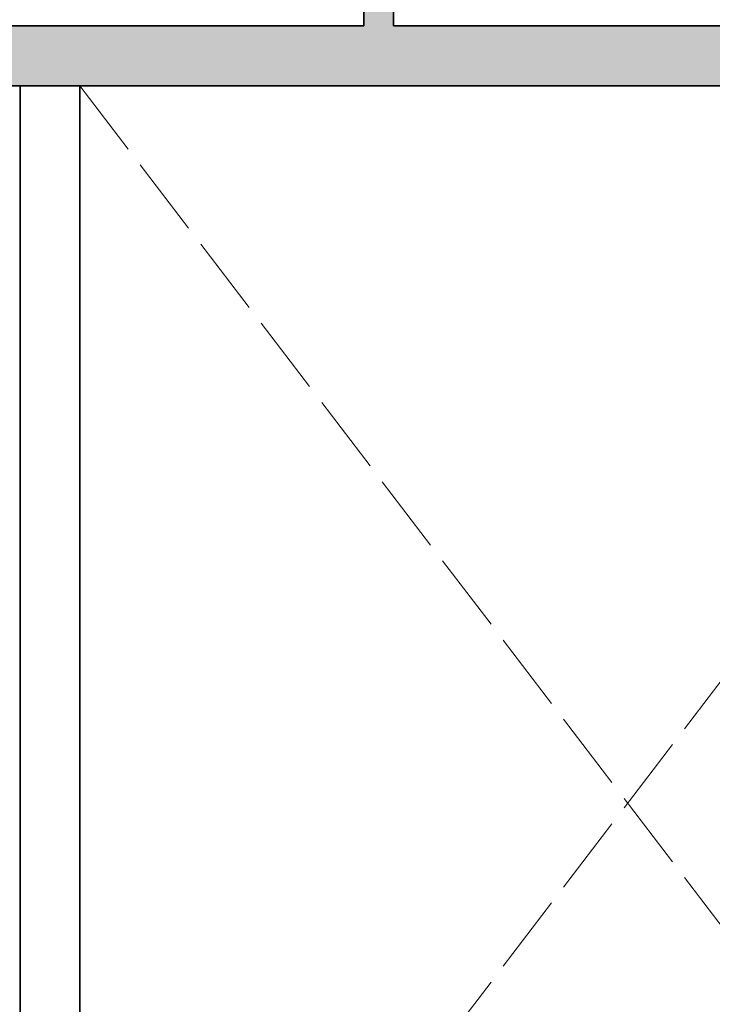
# Model space of a CAD drawing. Units: inches. Extents: x 2083 to 3317, y 1141 to 2115.
# Tile 252 of 256: x 2944 to 3048, y 1564 to 1713. Entities that reach past the tile are written whole.
import ezdxf

# ---------------------------------------------------------------- set-up
doc = ezdxf.new("R2010")
doc.units = ezdxf.units.IN
doc.linetypes.add('ACAD_ISO02W100', pattern=[15, 12, -3])
for name, color, linetype, lineweight in [('A-ANNO-DIMS', 2, 'Continuous', 18), ('A-FLOR-OPEN', 8, 'ACAD_ISO02W100', 13), ('A-WALL', 7, 'Continuous', 35)]:
    doc.layers.add(name, color=color, linetype=linetype, lineweight=lineweight)
doc.layers.add('A-WALL-PATT', color=251, linetype='Continuous', lineweight=13, true_color=0x636466)
doc.styles.get("Standard").update_dxf_attribs({"font": 'arial.ttf'})
doc.dimstyles.new('ISO-25', dxfattribs={"dimtxt": 12, "dimasz": 12, "dimexe": 1.25, "dimexo": 0.625, "dimtad": 1, "dimlunit": 3, "dimtxsty": 'Standard', "dimcen": 2.5, "dimadec": 0, "dimazin": 0, "dimtfac": 1, "dimtmove": 0, "dimatfit": 3, "dimfxl": 1, "dimarcsym": 0})

# ---------------------------------------------------------------- blocks, each defined once
blk = doc.blocks.new('*D71')
at = {"layer": 'A-ANNO-DIMS', "color": 0, "lineweight": -2, "transparency": 16777216}
for p, q in [((2997.14, 1794.66), (3020.88, 1769.53)), ((3093.61, 1692.52), (3029.12, 1760.8))]:
    blk.add_line(p, q, dxfattribs=at)
at = {"layer": 'A-ANNO-DIMS', "color": 0, "transparency": 16777216}
blk.add_solid([(3030.57, 1762.18), (3027.67, 1759.43), (3020.88, 1769.53)], dxfattribs=at)
at = {"layer": 'Defpoints', "color": 0, "transparency": 16777216}
for p in [(2997.14, 1794.66), (3020.88, 1769.53)]:
    blk.add_point(p, dxfattribs=at)
at = {"layer": 'A-ANNO-DIMS', "color": 0, "transparency": 16777216, "insert": (3070.45, 1726.99), "char_height": 12, "attachment_point": 5, "rotation": 313.3638}
blk.add_mtext('R2\'-10 1/2"', dxfattribs=at)

msp = doc.modelspace()

# ---------------------------------------------------------------- hatches: boundary and pattern name
at = {"layer": 'A-WALL-PATT'}
h = msp.add_hatch(color=256, dxfattribs=at)
h.dxf.hatch_style = 1
h.paths.add_polyline_path([(3126.96, 2020.761), (2748.96, 2020.761), (2604.96, 2020.761), (2226.96, 2020.761), (2226.96, 1702.761), (2466.96, 1702.761), (2466.96, 1582.761), (2418.96, 1582.761), (2418.96, 1477.761), (2226.96, 1477.761), (2226.96, 1263.261), (2544.96, 1263.261), (2544.96, 1411.761), (2604.96, 1411.761), (2685.96, 1411.761), (2685.96, 1420.761), (2604.96, 1420.761), (2604.96, 1573.761), (2604.96, 1702.761), (2604.96, 2011.761), (2748.96, 2011.761), (2748.96, 1702.761), (2862.96, 1702.761), (2862.96, 1621.761), (2871.96, 1621.761), (2871.96, 1702.761), (2883.96, 1702.761), (2883.96, 1706.939, -0.0264593), (2883.96, 1711.761), (2757.96, 1711.761), (2757.96, 1807.761), (2787.96, 1807.761), (2787.96, 1812.261), (2757.96, 1812.261), (2757.96, 2011.761), (2877.96, 2011.761), (2877.96, 1812.261), (2847.96, 1812.261), (2847.96, 1807.761), (2889.836, 1807.761), (2889.836, 1812.261), (2882.46, 1812.261), (2882.46, 2011.761), (3117.96, 2011.761), (3117.96, 1812.261), (2937.836, 1812.261), (2937.836, 1807.761), (2995.71, 1807.761), (2995.71, 1796.118), (3000.21, 1796.118), (3000.21, 1807.761), (3117.96, 1807.761), (3117.96, 1711.761), (3000.21, 1711.761), (3000.21, 1760.118), (2998.573, 1760.118, -0.020711), (2995.71, 1760.118), (2995.71, 1711.761), (2931.96, 1711.761), (2931.96, 1702.761), (3126.96, 1702.761)])
h.paths.add_polyline_path([(2471.46, 2011.761), (2471.46, 1810.011), (2462.717, 1810.011), (2462.717, 1805.511), (2505.96, 1805.511), (2505.96, 1810.011), (2475.96, 1810.011), (2475.96, 2011.761), (2595.96, 2011.761), (2595.96, 1810.011), (2565.96, 1810.011), (2565.96, 1805.511), (2595.96, 1805.511), (2595.96, 1711.761), (2235.96, 1711.761), (2235.96, 1805.511), (2353.71, 1805.511), (2353.71, 1796.054), (2358.21, 1796.054), (2358.21, 1805.511), (2414.717, 1805.511), (2414.717, 1810.011), (2235.96, 1810.011), (2235.96, 2011.761)], flags=16)
h.paths.add_polyline_path([(2270.205, 1994.61), (2270.205, 1970.61), (2246.205, 1970.61), (2246.205, 1994.61)], flags=0)
edge = h.paths.add_edge_path(flags=0)
edge.add_ellipse((2332.027, 1899.798), major_axis=(-3.043, 3.043), ratio=0.1682525, start_angle=-161.33217, end_angle=-156.30711, ccw=False)
edge.add_ellipse((2333.082, 1898.744), major_axis=(-1.055, 1.055), ratio=0.4535321, start_angle=-123.37102, end_angle=-94.15911)
edge = h.paths.add_edge_path(flags=0)
edge.add_ellipse((2332.027, 1968.876), major_axis=(3.043, 3.043), ratio=0.1682525, start_angle=18.66783, end_angle=23.69289)
edge.add_spline(control_points=[(2332.926, 1970.691), (2332.227, 1970.336), (2330.894, 1969.659), (2328.413, 1970.932), (2327.204, 1967.749), (2324.71, 1969.956), (2322.533, 1967.012), (2320.013, 1971.296), (2317.68, 1968.158), (2316.041, 1967.102), (2315.427, 1966.81)], knot_values=[0, 0, 0, 0, 2.2670587, 4.3245589, 6.6855835, 8.8786411, 11.121502, 14.300359, 17.7552837, 19.732645, 19.732645, 19.732645, 19.732645], degree=3, periodic=0)
edge.add_ellipse((2332.027, 1968.876), major_axis=(3.043, 3.043), ratio=0.1682525, start_angle=18.66783, end_angle=23.69289, ccw=False)
edge.add_ellipse((2333.082, 1969.931), major_axis=(1.055, 1.055), ratio=0.4535321, start_angle=56.62898, end_angle=85.84089, ccw=False)
edge = h.paths.add_edge_path(flags=0)
edge.add_spline(control_points=[(2296.428, 1967.988), (2293.628, 1965.336), (2287.704, 1959.727), (2299.744, 1949.996), (2294.533, 1935.669), (2290.573, 1920.604), (2293.394, 1909.974), (2296.185, 1904.967)], knot_values=[0.0991853, 0.0991853, 0.0991853, 0.0991853, 0.3453009, 0.6198217, 0.9826526, 1.3860932, 1.8105546, 1.8105546, 1.8105546, 1.8105546], degree=3, periodic=0)
edge.add_spline(control_points=[(2296.185, 1904.967), (2297.384, 1902.619), (2298.001, 1901.949), (2298.553, 1901.468)], knot_values=[0.0062457, 0.0062457, 0.0062457, 0.0062457, 0.0554759, 0.0554759, 0.0554759, 0.0554759], degree=3, periodic=0)
edge.add_spline(control_points=[(2298.553, 1901.468), (2297.259, 1900.923), (2295.225, 1900.232), (2293.06, 1900.614), (2292.101, 1900.788), (2292.09, 1900.791)], knot_values=[0.3128349, 0.3128349, 0.3128349, 0.3128349, 0.4017797, 0.4749867, 0.4759027, 0.4759027, 0.4759027, 0.4759027], degree=3, periodic=0)
edge.add_arc((2292.794, 1904.664), 3.937, 215.4209, 259.69818, ccw=False)
edge.add_spline(control_points=[(2289.585, 1902.382), (2289.477, 1902.535), (2289.368, 1902.688), (2289.261, 1902.841)], knot_values=[0.1028719, 0.1028719, 0.1028719, 0.1028719, 0.1168958, 0.1168958, 0.1168958, 0.1168958], degree=3, periodic=0)
edge.add_spline(control_points=[(2289.261, 1902.841), (2288.687, 1902.55), (2287.64, 1902.02), (2285.881, 1901.874), (2283.853, 1901.504), (2281.72, 1899.711), (2278.467, 1899.493), (2276.157, 1901.883), (2272.259, 1899.804), (2267.778, 1901.843), (2262.244, 1900.184), (2257.415, 1901.782), (2254.318, 1900.726), (2253.178, 1900.337)], knot_values=[0, 0, 0, 0, 1.9079767, 3.4771759, 5.261074, 7.9728515, 11.6802485, 13.7179214, 16.9395917, 22.789562, 27.5025027, 33.5952153, 37.1456181, 37.1456181, 37.1456181, 37.1456181], degree=3, periodic=0)
edge.add_line((2253.178, 1900.337), (2250.244, 1902.841))
edge.add_line((2250.244, 1902.841), (2250.244, 1965.833))
edge.add_line((2250.244, 1965.833), (2253.178, 1968.337))
edge.add_spline(control_points=[(2253.178, 1968.337), (2254.318, 1967.948), (2257.415, 1966.892), (2262.244, 1968.49), (2267.778, 1966.831), (2271.527, 1968.537), (2273.876, 1967.828), (2274.207, 1967.728)], knot_values=[0, 0, 0, 0, 0.0901802, 0.2449351, 0.3646438, 0.5132331, 0.5378548, 0.5378548, 0.5378548, 0.5378548], degree=3, periodic=0)
edge.add_arc((2274.353, 1963.793), 3.937, 72.05113, 92.12795, ccw=False)
edge.add_arc((2281.297, 1985.23), 18.596, 252.05113, 288.56572)
edge.add_arc((2292.317, 1956.029), 12.646, 71.02679, 113.77822, ccw=False)
edge = h.paths.add_edge_path(flags=0)
edge.add_spline(control_points=[(2274.899, 1951.856), (2275.066, 1951.617), (2275.233, 1951.377), (2275.398, 1951.136)], knot_values=[1.4099157, 1.4099157, 1.4099157, 1.4099157, 1.4315903, 1.4315903, 1.4315903, 1.4315903], degree=3, periodic=0)
edge.add_spline(control_points=[(2275.398, 1951.136), (2275.792, 1950.562), (2276.179, 1949.984), (2276.546, 1949.397)], knot_values=[1.3582378, 1.3582378, 1.3582378, 1.3582378, 1.4099157, 1.4099157, 1.4099157, 1.4099157], degree=3, periodic=0)
edge.add_line((2276.546, 1949.397), (2277.437, 1947.862))
edge.add_spline(control_points=[(2277.437, 1947.862), (2276.304, 1945.673), (2274.64, 1942.427), (2274.632, 1938.094), (2272.799, 1930.852), (2274.356, 1943.897), (2275.948, 1947.923), (2276.546, 1949.397)], knot_values=[0.0056315, 0.0056315, 0.0056315, 0.0056315, 0.1860139, 0.2660015, 0.3570872, 0.5963902, 0.7397317, 0.7397317, 0.7397317, 0.7397317], degree=3, periodic=0)
edge.add_spline(control_points=[(2276.546, 1949.397), (2276.179, 1949.984), (2275.792, 1950.562), (2275.398, 1951.136)], knot_values=[1.3582378, 1.3582378, 1.3582378, 1.3582378, 1.4099157, 1.4099157, 1.4099157, 1.4099157], degree=3, periodic=0)
edge.add_spline(control_points=[(2275.398, 1951.136), (2274.943, 1950.08), (2274.208, 1948.025), (2273.935, 1944.851), (2272.469, 1937.627), (2273.466, 1945.696), (2274.701, 1951.059), (2274.899, 1951.856)], knot_values=[0.1043639, 0.1043639, 0.1043639, 0.1043639, 0.1896363, 0.2696239, 0.3607096, 0.6000126, 0.6446217, 0.6446217, 0.6446217, 0.6446217], degree=3, periodic=0)
h.paths.add_polyline_path([(2269.168, 1963.128, -0.3575267), (2268.171, 1960.976, -0.0925607), (2268.171, 1939.436, -0.3575267), (2269.168, 1937.285, -0.3575267), (2267.016, 1938.282, -0.1647847), (2254.686, 1938.282, -0.3575267), (2252.534, 1937.285, -0.3575267), (2253.531, 1939.436, -0.0925607), (2253.531, 1960.976, -0.3575267), (2252.534, 1963.128, -0.3575267), (2254.686, 1962.131, -0.1647847), (2267.016, 1962.131, -0.3575267)], flags=0)
h.paths.add_polyline_path([(2248.874, 1967.802), (2248.874, 1957.028), (2249.458, 1957.028), (2249.458, 1911.647), (2248.874, 1911.647), (2248.874, 1900.873), (2246.512, 1900.873, 0.1973271), (2244.15, 1902.457), (2244.15, 1966.218, 0.1973271), (2246.512, 1967.802)], flags=0)
h.paths.add_polyline_path([(2269.168, 1931.389, -0.3575267), (2268.171, 1929.238, -0.0925607), (2268.171, 1907.698, -0.3575267), (2269.168, 1905.547, -0.3575267), (2267.016, 1906.544, -0.1647847), (2254.686, 1906.544, -0.3575267), (2252.534, 1905.547, -0.3575267), (2253.531, 1907.698, -0.0925607), (2253.531, 1929.238, -0.3575267), (2252.534, 1931.389, -0.3575267), (2254.686, 1930.392, -0.1647847), (2267.016, 1930.392, -0.3575267)], flags=0)
edge = h.paths.add_edge_path(flags=0)
edge.add_spline(control_points=[(2276.197, 1906.724), (2276.168, 1909.029), (2276.114, 1913.372), (2270.598, 1924.925), (2273.905, 1919.013), (2275.922, 1916.262), (2275.475, 1912.402), (2277.258, 1910.381), (2276.696, 1908.225), (2276.646, 1906.813), (2276.618, 1906.008)], knot_values=[0, 0, 0, 0, 8.6102597, 16.2212739, 18.8430575, 23.8048978, 27.4408283, 29.3561016, 31.2034776, 33.6506866, 33.6506866, 33.6506866, 33.6506866], degree=3, periodic=0)
edge.add_spline(control_points=[(2276.618, 1906.008), (2276.623, 1905.624), (2276.498, 1904.629), (2275.442, 1903.855), (2274.937, 1903.08), (2274.859, 1902.841)], knot_values=[0.1564884, 0.1564884, 0.1564884, 0.1564884, 0.1843975, 0.2313765, 0.2505985, 0.2505985, 0.2505985, 0.2505985], degree=3, periodic=0)
edge.add_line((2274.859, 1902.841), (2276.506, 1902.841))
edge.add_spline(control_points=[(2276.506, 1902.841), (2276.788, 1903.085), (2277.665, 1904.125), (2278.25, 1904.341), (2277.654, 1908.527), (2278.156, 1906.228), (2278.1, 1905.286), (2278.847, 1904.069), (2277.857, 1903.415), (2277.874, 1902.991), (2277.904, 1902.841)], knot_values=[0.0595743, 0.0595743, 0.0595743, 0.0595743, 0.0807529, 0.1037415, 0.1697201, 0.1760361, 0.2071372, 0.2404744, 0.2623409, 0.2736605, 0.2736605, 0.2736605, 0.2736605], degree=3, periodic=0)
edge.add_line((2277.904, 1902.841), (2280.03, 1902.841))
edge.add_spline(control_points=[(2280.03, 1902.841), (2279.888, 1903.088), (2279.499, 1903.982), (2280.152, 1905.939), (2278.104, 1909.658), (2279.762, 1907.185), (2280.328, 1904.875), (2280.485, 1903.49), (2281.463, 1903.249), (2281.758, 1902.936), (2281.834, 1902.841)], knot_values=[0.013856, 0.013856, 0.013856, 0.013856, 0.0348738, 0.0888667, 0.1078792, 0.1267378, 0.158714, 0.1937575, 0.2174868, 0.2267221, 0.2267221, 0.2267221, 0.2267221], degree=3, periodic=0)
edge.add_spline(control_points=[(2281.834, 1902.841), (2281.788, 1902.827), (2281.647, 1902.783), (2281.396, 1902.859), (2281.088, 1902.985), (2280.721, 1903.061), (2280.333, 1903.026), (2280.125, 1902.899), (2280.03, 1902.841)], knot_values=[0, 0, 0, 0, 0.1441304, 0.435517, 0.7492759, 1.1530457, 1.5483707, 1.878348, 1.878348, 1.878348, 1.878348], degree=3, periodic=0)
edge.add_line((2280.03, 1902.841), (2277.904, 1902.841))
edge.add_spline(control_points=[(2277.904, 1902.841), (2277.893, 1902.796), (2277.865, 1902.68), (2277.607, 1902.687), (2277.274, 1902.801), (2276.838, 1902.62), (2276.584, 1902.789), (2276.506, 1902.841)], knot_values=[0, 0, 0, 0, 0.1271885, 0.3261988, 0.6280094, 1.2435704, 1.5153306, 1.5153306, 1.5153306, 1.5153306], degree=3, periodic=0)
edge.add_line((2276.506, 1902.841), (2274.859, 1902.841))
edge.add_spline(control_points=[(2274.859, 1902.841), (2274.814, 1902.899), (2274.725, 1903.013), (2274.493, 1903.119), (2274.244, 1902.961), (2273.937, 1903.185), (2273.614, 1902.983), (2273.408, 1902.883), (2273.322, 1902.841)], knot_values=[0, 0, 0, 0, 0.2184302, 0.4369566, 0.6879766, 0.9903786, 1.3983955, 1.6918498, 1.6918498, 1.6918498, 1.6918498], degree=3, periodic=0)
edge.add_spline(control_points=[(2273.322, 1902.841), (2273.617, 1903.446), (2274.274, 1904.538), (2276.027, 1904.574), (2276.207, 1906.584), (2276.197, 1906.724)], knot_values=[0.0122268, 0.0122268, 0.0122268, 0.0122268, 0.0594721, 0.1062177, 0.134458, 0.134458, 0.134458, 0.134458], degree=3, periodic=0)
h.paths.add_polyline_path([(2270.776, 1897.79), (2270.776, 1873.79), (2246.776, 1873.79), (2246.776, 1897.79)], flags=0)
h.paths.add_polyline_path([(2353.71, 1760.005), (2353.71, 1760.054), (2358.21, 1760.054, -0.033729)], flags=0)
h.paths.add_polyline_path([(2321.819, 1737.529), (2341.995, 1737.529, -0.4142136), (2343.203, 1736.321), (2343.203, 1721.021, -0.4142136), (2341.995, 1719.813), (2321.819, 1719.813, -0.4142136), (2320.611, 1721.021), (2320.611, 1736.321, -0.4142136)], flags=0)
h.paths.add_polyline_path([(2324.235, 1736.321), (2339.579, 1736.321, -0.4142136), (2341.995, 1733.905), (2341.995, 1725.45, -0.4142136), (2339.579, 1723.034), (2333.681, 1723.034), (2333.845, 1722.045, -0.8706461), (2335.425, 1721.826, -0.767327), (2333.923, 1721.423), (2331.291, 1721.423, -0.767327), (2329.788, 1721.826, -0.8706461), (2331.368, 1722.045), (2331.533, 1723.034), (2324.235, 1723.034, -0.4142136), (2321.819, 1725.45), (2321.819, 1733.905, -0.4142136)], flags=0)
h.paths.add_polyline_path([(2570.484, 1928.615), (2589.684, 1928.615), (2590.169, 1928.615), (2590.169, 1904.993), (2570.484, 1904.993)], flags=0)
h.paths.add_polyline_path([(2574.447, 1927.264, -1), (2572.829, 1927.264, -1)], flags=0)
h.paths.add_polyline_path([(2573.09, 1926.941), (2573.925, 1927.776), (2574.148, 1927.553), (2573.313, 1926.718)], flags=0)
h.paths.add_polyline_path([(2578.779, 1919.73, -1), (2571.592, 1919.73, -1)], flags=0)
h.paths.add_polyline_path([(2578.385, 1919.73, -1), (2571.985, 1919.73, -1)], flags=0)
h.paths.add_polyline_path([(2331.596, 1729.476, -1), (2333.618, 1729.476, -1)], flags=0)
h.paths.add_polyline_path([(2578.034, 1927.264, -1), (2576.416, 1927.264, -1)], flags=0)
h.paths.add_polyline_path([(2576.689, 1927.531), (2576.912, 1927.754), (2577.747, 1926.919), (2577.524, 1926.696)], flags=0)
h.paths.add_polyline_path([(2578.139, 1909.86, -1), (2572.232, 1909.86, -1)], flags=0)
h.paths.add_polyline_path([(2577.745, 1909.86, -1), (2572.625, 1909.86, -1)], flags=0)
h.paths.add_polyline_path([(2583.798, 1927.264, -1), (2582.179, 1927.264, -1)], flags=0)
h.paths.add_polyline_path([(2582.719, 1927.754), (2583.554, 1926.919), (2583.331, 1926.696), (2582.496, 1927.531)], flags=0)
h.paths.add_polyline_path([(2582.496, 1927.531), (2582.719, 1927.754), (2583.554, 1926.919), (2583.331, 1926.696)], flags=0)
h.paths.add_polyline_path([(2587.739, 1920.53, -1), (2581.832, 1920.53, -1)], flags=0)
h.paths.add_polyline_path([(2587.345, 1920.53, -1), (2582.225, 1920.53, -1)], flags=0)
h.paths.add_polyline_path([(2587.385, 1927.264, -1), (2585.766, 1927.264, -1)], flags=0)
h.paths.add_polyline_path([(2586.082, 1926.98), (2586.917, 1927.815), (2587.14, 1927.593), (2586.305, 1926.758)], flags=0)
h.paths.add_polyline_path([(2588.379, 1910.66, -1), (2581.192, 1910.66, -1)], flags=0)
h.paths.add_polyline_path([(2587.985, 1910.66, -1), (2581.585, 1910.66, -1)], flags=0)
h.paths.add_polyline_path([(2417.168, 1729.478), (2437.344, 1729.478, -0.4142136), (2438.552, 1728.27), (2438.552, 1712.969, -0.4142136), (2437.344, 1711.761), (2417.168, 1711.761, -0.4142136), (2415.96, 1712.969), (2415.96, 1728.27, -0.4142136)], flags=0)
h.paths.add_polyline_path([(2419.584, 1728.27), (2434.928, 1728.27, -0.4142136), (2437.344, 1725.854), (2437.344, 1717.398, -0.4142136), (2434.928, 1714.983), (2429.029, 1714.983), (2429.194, 1713.994, -0.8706461), (2430.774, 1713.775, -0.767327), (2429.271, 1713.372), (2426.64, 1713.372, -0.767327), (2425.137, 1713.775, -0.8706461), (2426.717, 1713.994), (2426.882, 1714.983), (2419.584, 1714.983, -0.4142136), (2417.168, 1717.398), (2417.168, 1725.854, -0.4142136)], flags=0)
h.paths.add_polyline_path([(2419.584, 1728.27), (2434.928, 1728.27, -0.4142136), (2437.344, 1725.854), (2437.344, 1717.398, -0.4142136), (2434.928, 1714.983), (2429.029, 1714.983), (2428.358, 1719.009), (2427.553, 1719.009), (2426.882, 1714.983), (2419.584, 1714.983, -0.4142136), (2417.168, 1717.398), (2417.168, 1725.854, -0.4142136)], flags=0)
h.paths.add_polyline_path([(2426.944, 1721.425, -1), (2428.967, 1721.425, -1)], flags=0)
h.paths.add_polyline_path([(2475.96, 1702.761), (2595.96, 1702.761), (2595.96, 1582.761), (2475.96, 1582.761)], flags=16)
h.paths.add_polyline_path([(2427.96, 1573.761), (2595.96, 1573.761), (2595.96, 1468.761), (2595.96, 1420.761), (2384.46, 1420.761), (2384.46, 1468.761), (2427.96, 1468.761)], flags=16)
h.paths.add_polyline_path([(2379.96, 1468.761), (2379.96, 1420.761), (2235.96, 1420.761), (2235.96, 1468.761)], flags=16)
h.paths.add_polyline_path([(2317.816, 1466.696), (2337.992, 1466.696, -0.4142136), (2339.2, 1465.488), (2339.2, 1450.187, -0.4142136), (2337.992, 1448.979), (2317.816, 1448.979, -0.4142136), (2316.608, 1450.187), (2316.608, 1465.488, -0.4142136)], flags=0)
h.paths.add_polyline_path([(2320.232, 1465.488), (2335.576, 1465.488, -0.4142136), (2337.992, 1463.072), (2337.992, 1454.616, -0.4142136), (2335.576, 1452.2), (2329.677, 1452.2), (2329.842, 1451.212, -0.8706461), (2331.422, 1450.992, -0.767327), (2329.92, 1450.59), (2327.288, 1450.59, -0.767327), (2325.785, 1450.992, -0.8706461), (2327.365, 1451.212), (2327.53, 1452.2), (2320.232, 1452.2, -0.4142136), (2317.816, 1454.616), (2317.816, 1463.072, -0.4142136)], flags=0)
h.paths.add_polyline_path([(2320.232, 1465.488), (2335.576, 1465.488, -0.4142136), (2337.992, 1463.072), (2337.992, 1454.616, -0.4142136), (2335.576, 1452.2), (2329.677, 1452.2), (2329.006, 1456.227), (2328.201, 1456.227), (2327.53, 1452.2), (2320.232, 1452.2, -0.4142136), (2317.816, 1454.616), (2317.816, 1463.072, -0.4142136)], flags=0)
h.paths.add_polyline_path([(2327.593, 1458.643, -1), (2329.615, 1458.643, -1)], flags=0)
h.paths.add_polyline_path([(2244.412, 1433.34), (2241.921, 1433.34, -0.4142136), (2240.018, 1435.244), (2240.018, 1440.953, -0.4142105), (2241.921, 1442.856), (2244.412, 1442.856, -1.9764724)], flags=0)
h.paths.add_polyline_path([(2245.357, 1434.398, -0.4142136), (2245.357, 1441.799, -2.1440985)], flags=0)
h.paths.add_polyline_path([(2535.96, 1416.261), (2535.96, 1272.261), (2235.96, 1272.261), (2235.96, 1416.261)], flags=16)
h.paths.add_polyline_path([(2260.12, 1384.293), (2260.12, 1362.039), (2237.865, 1362.039), (2237.865, 1384.293)], flags=0)
edge = h.paths.add_edge_path(flags=0)
edge.add_line((2318.252, 1362.093), (2318.146, 1362.001))
edge.add_ellipse((2317.445, 1360.431), major_axis=(2.822, 2.822), ratio=0.1682525, start_angle=18.66783, end_angle=20.94813, ccw=False)
edge.add_ellipse((2318.423, 1361.409), major_axis=(0.978, 0.978), ratio=0.4535321, start_angle=56.62898, end_angle=70.2262, ccw=False)
edge = h.paths.add_edge_path(flags=0)
edge.add_line((2319.107, 1295.571), (2319.015, 1295.677))
edge.add_ellipse((2317.445, 1296.378), major_axis=(-2.822, 2.822), ratio=0.1682525, start_angle=-161.33217, end_angle=-159.05187, ccw=False)
edge.add_ellipse((2318.423, 1295.4), major_axis=(-0.978, 0.978), ratio=0.4535321, start_angle=-123.37102, end_angle=-109.7738)
edge = h.paths.add_edge_path(flags=0)
edge.add_spline(control_points=[(2284.21, 1301.17), (2284.581, 1300.445), (2284.891, 1299.892), (2285.16, 1299.461)], knot_values=[0.0390658, 0.0390658, 0.0390658, 0.0390658, 0.0554759, 0.0554759, 0.0554759, 0.0554759], degree=3, periodic=0)
edge.add_line((2285.16, 1299.461), (2284.21, 1301.17))
edge = h.paths.add_edge_path(flags=0)
edge.add_line((2280.412, 1297.298), (2283.37, 1297.036))
edge.add_line((2283.37, 1297.036), (2286.406, 1297.926))
edge.add_spline(control_points=[(2286.406, 1297.926), (2285.305, 1297.463), (2284.345, 1297.129), (2283.37, 1297.036)], knot_values=[0.3943688, 0.3943688, 0.3943688, 0.3943688, 0.4759027, 0.4759027, 0.4759027, 0.4759027], degree=3, periodic=0)
edge.add_spline(control_points=[(2283.37, 1297.036), (2283.281, 1297.028), (2282.316, 1296.957), (2281.313, 1297.134), (2280.423, 1297.296), (2280.412, 1297.298)], knot_values=[0.3128349, 0.3128349, 0.3128349, 0.3128349, 0.3202458, 0.3934528, 0.3943688, 0.3943688, 0.3943688, 0.3943688], degree=3, periodic=0)
edge = h.paths.add_edge_path(flags=0)
edge.add_line((2284.436, 1359.607), (2280.446, 1355.328))
edge.add_line((2280.446, 1355.328), (2279.58, 1351.018))
edge.add_line((2279.58, 1351.018), (2282.413, 1346.58))
edge.add_spline(control_points=[(2282.413, 1346.58), (2283.153, 1345.589), (2284.253, 1344.029), (2284.801, 1342.387), (2284.935, 1341.806)], knot_values=[1.2400982, 1.2400982, 1.2400982, 1.2400982, 1.3328922, 1.3827123, 1.3827123, 1.3827123, 1.3827123], degree=3, periodic=0)
edge.add_spline(control_points=[(2284.935, 1341.806), (2285.319, 1340.141), (2285.233, 1338.409), (2284.91, 1336.654)], knot_values=[1.0974841, 1.0974841, 1.0974841, 1.0974841, 1.2400982, 1.2400982, 1.2400982, 1.2400982], degree=3, periodic=0)
edge.add_spline(control_points=[(2284.91, 1336.654), (2284.587, 1334.899), (2284.027, 1333.12), (2283.463, 1331.361)], knot_values=[0.9548699, 0.9548699, 0.9548699, 0.9548699, 1.0974841, 1.0974841, 1.0974841, 1.0974841], degree=3, periodic=0)
edge.add_line((2283.463, 1331.361), (2281.89, 1326.153))
edge.add_line((2281.89, 1326.153), (2280.756, 1321.056))
edge.add_line((2280.756, 1321.056), (2280.299, 1316.002))
edge.add_line((2280.299, 1316.002), (2280.716, 1310.95))
edge.add_line((2280.716, 1310.95), (2282.028, 1305.972))
edge.add_line((2282.028, 1305.972), (2284.21, 1301.17))
edge.add_spline(control_points=[(2284.21, 1301.17), (2283.341, 1302.73), (2282.612, 1304.336), (2282.028, 1305.972)], knot_values=[0.0991853, 0.0991853, 0.0991853, 0.0991853, 0.2417994, 0.2417994, 0.2417994, 0.2417994], degree=3, periodic=0)
edge.add_spline(control_points=[(2282.028, 1305.972), (2281.444, 1307.608), (2281.005, 1309.273), (2280.716, 1310.95)], knot_values=[0.2417994, 0.2417994, 0.2417994, 0.2417994, 0.3844135, 0.3844135, 0.3844135, 0.3844135], degree=3, periodic=0)
edge.add_spline(control_points=[(2280.716, 1310.95), (2280.433, 1312.588), (2280.289, 1314.277), (2280.299, 1315.962), (2280.299, 1316.002)], knot_values=[0.3844135, 0.3844135, 0.3844135, 0.3844135, 0.5236467, 0.5270276, 0.5270276, 0.5270276, 0.5270276], degree=3, periodic=0)
edge.add_spline(control_points=[(2280.299, 1316.002), (2280.312, 1317.687), (2280.478, 1319.368), (2280.756, 1321.056)], knot_values=[0.5270276, 0.5270276, 0.5270276, 0.5270276, 0.6696417, 0.6696417, 0.6696417, 0.6696417], degree=3, periodic=0)
edge.add_spline(control_points=[(2280.756, 1321.056), (2281.035, 1322.744), (2281.426, 1324.44), (2281.89, 1326.153)], knot_values=[0.6696417, 0.6696417, 0.6696417, 0.6696417, 0.8122558, 0.8122558, 0.8122558, 0.8122558], degree=3, periodic=0)
edge.add_spline(control_points=[(2281.89, 1326.153), (2282.264, 1327.533), (2282.788, 1329.262), (2283.353, 1331.018), (2283.463, 1331.361)], knot_values=[0.8122558, 0.8122558, 0.8122558, 0.8122558, 0.9270873, 0.9548699, 0.9548699, 0.9548699, 0.9548699], degree=3, periodic=0)
edge.add_line((2283.463, 1331.361), (2284.91, 1336.654))
edge.add_line((2284.91, 1336.654), (2284.935, 1341.806))
edge.add_line((2284.935, 1341.806), (2282.413, 1346.58))
edge.add_spline(control_points=[(2282.413, 1346.58), (2281.275, 1348.104), (2280.078, 1349.57), (2279.58, 1351.018)], knot_values=[1.3827123, 1.3827123, 1.3827123, 1.3827123, 1.5253264, 1.5253264, 1.5253264, 1.5253264], degree=3, periodic=0)
edge.add_spline(control_points=[(2279.58, 1351.018), (2279.443, 1351.415), (2279.136, 1352.857), (2279.735, 1354.29), (2280.446, 1355.328)], knot_values=[1.5253264, 1.5253264, 1.5253264, 1.5253264, 1.564439, 1.6679405, 1.6679405, 1.6679405, 1.6679405], degree=3, periodic=0)
edge.add_spline(control_points=[(2280.446, 1355.328), (2281.426, 1356.758), (2282.931, 1358.183), (2284.436, 1359.607)], knot_values=[1.6679405, 1.6679405, 1.6679405, 1.6679405, 1.8105546, 1.8105546, 1.8105546, 1.8105546], degree=3, periodic=0)
edge.add_arc((2280.623, 1348.518), 11.726, 71.02679, 113.77822)
edge.add_arc((2270.405, 1375.595), 17.244, 252.05113, 288.56572, ccw=False)
edge.add_arc((2263.966, 1355.718), 3.651, 72.05113, 92.12795)
edge.add_arc((2263.966, 1355.718), 3.651, 92.12795, 177.98513)
edge.add_spline(control_points=[(2260.318, 1355.846), (2260.26, 1354.221), (2260.551, 1350.187), (2262.999, 1346.766), (2264.473, 1344.649)], knot_values=[1.4315903, 1.4315903, 1.4315903, 1.4315903, 1.5641438, 1.7706953, 1.7706953, 1.7706953, 1.7706953], degree=3, periodic=0)
edge.add_line((2264.473, 1344.649), (2264.936, 1343.983))
edge.add_spline(control_points=[(2263.801, 1340.248), (2263.843, 1340.514), (2264.067, 1341.756), (2264.513, 1343.002), (2264.935, 1343.981)], knot_values=[0.5365702, 0.5365702, 0.5365702, 0.5365702, 0.5593494, 0.6446217, 0.6446217, 0.6446217, 0.6446217], degree=3, periodic=0)
edge.add_spline(control_points=[(2264.935, 1343.981), (2265.118, 1343.715), (2265.299, 1343.448), (2265.477, 1343.179)], knot_values=[1.3840767, 1.3840767, 1.3840767, 1.3840767, 1.4099157, 1.4099157, 1.4099157, 1.4099157], degree=3, periodic=0)
edge.add_spline(control_points=[(2265.477, 1343.179), (2265.655, 1342.911), (2265.829, 1342.641), (2265.999, 1342.369)], knot_values=[1.3582378, 1.3582378, 1.3582378, 1.3582378, 1.3840767, 1.3840767, 1.3840767, 1.3840767], degree=3, periodic=0)
edge.add_line((2265.999, 1342.369), (2266.826, 1340.946))
edge.add_spline(control_points=[(2266.826, 1340.946), (2268.894, 1337.09), (2271.398, 1325.843), (2270.516, 1310.569), (2275.919, 1301.861), (2277.79, 1299.199)], knot_values=[0.1168958, 0.1168958, 0.1168958, 0.1168958, 0.4729873, 1.0509689, 1.3137934, 1.3137934, 1.3137934, 1.3137934], degree=3, periodic=0)
edge.add_spline(control_points=[(2277.79, 1299.199), (2277.839, 1299.128), (2277.889, 1299.057), (2277.94, 1298.987)], knot_values=[0.1098839, 0.1098839, 0.1098839, 0.1098839, 0.1168958, 0.1168958, 0.1168958, 0.1168958], degree=3, periodic=0)
edge.add_line((2277.94, 1298.987), (2277.789, 1299.199))
edge.add_spline(control_points=[(2277.789, 1299.199), (2277.257, 1298.929), (2276.286, 1298.438), (2275.039, 1298.334), (2274.383, 1298.239), (2274.215, 1298.209)], knot_values=[33.1218702, 33.1218702, 33.1218702, 33.1218702, 35.0290557, 36.5982549, 37.1448269, 37.1448269, 37.1448269, 37.1448269], degree=3, periodic=0)
edge.add_line((2274.215, 1298.209), (2273.073, 1297.893))
edge.add_spline(control_points=[(2273.073, 1297.893), (2272.323, 1297.58), (2271.039, 1296.511), (2269.248, 1296.226), (2268.423, 1296.375)], knot_values=[26.5325843, 26.5325843, 26.5325843, 26.5325843, 29.198919, 31.8391012, 31.8391012, 31.8391012, 31.8391012], degree=3, periodic=0)
edge.add_line((2268.423, 1296.375), (2263.879, 1297.458))
edge.add_spline(control_points=[(2263.879, 1297.458), (2263.556, 1297.359), (2261.86, 1296.839), (2260.239, 1297.282), (2258.933, 1297.516)], knot_values=[15.9195506, 15.9195506, 15.9195506, 15.9195506, 16.9395917, 21.2260675, 21.2260675, 21.2260675, 21.2260675], degree=3, periodic=0)
edge.add_line((2258.933, 1297.516), (2254.055, 1297.329))
edge.add_spline(control_points=[(2254.055, 1297.329), (2253.756, 1297.296), (2252.114, 1297.165), (2250.462, 1297.544), (2249.13, 1297.668)], knot_values=[5.3065169, 5.3065169, 5.3065169, 5.3065169, 6.2764352, 10.6130337, 10.6130337, 10.6130337, 10.6130337], degree=3, periodic=0)
edge.add_line((2249.13, 1297.668), (2244.332, 1296.878))
edge.add_line((2244.332, 1296.878), (2241.611, 1299.199))
edge.add_line((2241.611, 1299.199), (2241.611, 1357.609))
edge.add_line((2241.611, 1357.609), (2244.332, 1359.931))
edge.add_line((2244.332, 1359.931), (2252.729, 1359.543))
edge.add_spline(control_points=[(2252.729, 1359.543), (2252.871, 1359.546), (2253.306, 1359.548), (2253.74, 1359.514), (2254.032, 1359.482)], knot_values=[0.233291, 0.233291, 0.233291, 0.233291, 0.2449351, 0.2689274, 0.2689274, 0.2689274, 0.2689274], degree=3, periodic=0)
edge.add_line((2254.032, 1359.482), (2259.587, 1359.416))
edge.add_spline(control_points=[(2259.587, 1359.416), (2260.677, 1359.629), (2262.073, 1359.897), (2263.524, 1359.459), (2263.83, 1359.366)], knot_values=[0.4225164, 0.4225164, 0.4225164, 0.4225164, 0.5132331, 0.5378548, 0.5378548, 0.5378548, 0.5378548], degree=3, periodic=0)
edge.add_arc((2263.966, 1355.718), 3.651, 72.05113, 92.12795, ccw=False)
edge.add_arc((2270.405, 1375.595), 17.244, 252.05113, 288.56572)
edge.add_arc((2280.623, 1348.518), 11.726, 71.02679, 113.77822, ccw=False)
h.paths.add_polyline_path([(2240.341, 1359.435), (2240.341, 1349.444), (2240.882, 1349.444), (2240.882, 1307.365), (2240.341, 1307.365), (2240.341, 1297.374), (2238.15, 1297.374, 0.1973271), (2235.96, 1298.843), (2235.96, 1357.966, 0.1973271), (2238.15, 1359.435)], flags=0)
h.paths.add_polyline_path([(2259.158, 1355.101, -0.3575267), (2258.233, 1353.106, -0.0925607), (2258.233, 1333.133, -0.3575267), (2259.158, 1331.138, -0.3575267), (2257.163, 1332.062, -0.1647847), (2245.729, 1332.062, -0.3575267), (2243.735, 1331.138, -0.3575267), (2244.659, 1333.133, -0.0925607), (2244.659, 1353.106, -0.3575267), (2243.735, 1355.101, -0.3575267), (2245.729, 1354.176, -0.1647847), (2257.163, 1354.176, -0.3575267)], flags=0)
edge = h.paths.add_edge_path(flags=0)
edge.add_line((2265.999, 1342.369), (2266.826, 1340.946))
edge.add_line((2266.826, 1340.946), (2265.308, 1337.814))
edge.add_line((2265.308, 1337.814), (2264.358, 1334.653))
edge.add_line((2264.358, 1334.653), (2264.262, 1333.8))
edge.add_spline(control_points=[(2264.262, 1333.8), (2264.208, 1333.187), (2264.162, 1332.366), (2264.007, 1331.414), (2263.969, 1331.202)], knot_values=[0.4644442, 0.4644442, 0.4644442, 0.4644442, 0.5166905, 0.5316081, 0.5316081, 0.5316081, 0.5316081], degree=3, periodic=0)
edge.add_spline(control_points=[(2263.969, 1331.202), (2263.775, 1330.119), (2263.424, 1328.791), (2263.257, 1328.531), (2263.234, 1328.515)], knot_values=[0.3726816, 0.3726816, 0.3726816, 0.3726816, 0.4488497, 0.4644442, 0.4644442, 0.4644442, 0.4644442], degree=3, periodic=0)
edge.add_spline(control_points=[(2263.234, 1328.515), (2263.096, 1328.42), (2263.131, 1329.301), (2263.275, 1330.616)], knot_values=[0.2809191, 0.2809191, 0.2809191, 0.2809191, 0.3726816, 0.3726816, 0.3726816, 0.3726816], degree=3, periodic=0)
edge.add_spline(control_points=[(2263.275, 1330.616), (2263.419, 1331.93), (2263.672, 1333.677), (2263.97, 1335.315)], knot_values=[0.1891566, 0.1891566, 0.1891566, 0.1891566, 0.2809191, 0.2809191, 0.2809191, 0.2809191], degree=3, periodic=0)
edge.add_spline(control_points=[(2263.97, 1335.315), (2264.1, 1336.032), (2264.419, 1337.622), (2264.755, 1338.864), (2264.947, 1339.491)], knot_values=[0.097394, 0.097394, 0.097394, 0.097394, 0.1375775, 0.1891566, 0.1891566, 0.1891566, 0.1891566], degree=3, periodic=0)
edge.add_spline(control_points=[(2264.947, 1339.491), (2265.29, 1340.606), (2265.644, 1341.494), (2265.999, 1342.369)], knot_values=[0.0056315, 0.0056315, 0.0056315, 0.0056315, 0.097394, 0.097394, 0.097394, 0.097394], degree=3, periodic=0)
h.paths.add_polyline_path([(2259.158, 1325.671, -0.3575267), (2258.233, 1323.676, -0.0925607), (2258.233, 1303.703, -0.3575267), (2259.158, 1301.708, -0.3575267), (2257.163, 1302.633, -0.1647847), (2245.729, 1302.633, -0.3575267), (2243.735, 1301.708, -0.3575267), (2244.659, 1303.703, -0.0925607), (2244.659, 1323.676, -0.3575267), (2243.735, 1325.671, -0.3575267), (2245.729, 1324.747, -0.1647847), (2257.163, 1324.747, -0.3575267)], flags=0)
edge = h.paths.add_edge_path(flags=0)
edge.add_spline(control_points=[(2261.709, 1317.311), (2261.679, 1317.418), (2261.762, 1317.389), (2262.491, 1316.09), (2262.962, 1315.301)], knot_values=[14.9558607, 14.9558607, 14.9558607, 14.9558607, 16.2212739, 18.6948259, 18.6948259, 18.6948259, 18.6948259], degree=3, periodic=0)
edge.add_spline(control_points=[(2262.962, 1315.301), (2262.99, 1315.254), (2263.702, 1314.067), (2264.349, 1313.127), (2264.73, 1312.164)], knot_values=[18.6948259, 18.6948259, 18.6948259, 18.6948259, 18.8430575, 22.433791, 22.433791, 22.433791, 22.433791], degree=3, periodic=0)
edge.add_spline(control_points=[(2264.73, 1312.164), (2264.876, 1311.796), (2265.177, 1310.77), (2265.143, 1309.559), (2265.248, 1308.824)], knot_values=[22.433791, 22.433791, 22.433791, 22.433791, 23.8048978, 26.1727562, 26.1727562, 26.1727562, 26.1727562], degree=3, periodic=0)
edge.add_line((2265.248, 1308.824), (2265.851, 1307.172))
edge.add_spline(control_points=[(2265.851, 1307.172), (2266.065, 1306.822), (2266.384, 1306.332), (2266.424, 1305.781), (2266.42, 1305.611)], knot_values=[28.0625624, 28.0625624, 28.0625624, 28.0625624, 29.3561016, 29.9117214, 29.9117214, 29.9117214, 29.9117214], degree=3, periodic=0)
edge.add_spline(control_points=[(2266.42, 1305.611), (2266.416, 1305.433), (2266.394, 1305.25), (2266.365, 1305.066)], knot_values=[29.9117214, 29.9117214, 29.9117214, 29.9117214, 30.4978371, 30.4978371, 30.4978371, 30.4978371], degree=3, periodic=0)
edge.add_line((2266.365, 1305.066), (2266.066, 1302.136))
edge.add_spline(control_points=[(2266.066, 1302.136), (2266.071, 1301.78), (2265.998, 1301.2), (2265.663, 1300.759), (2265.509, 1300.586)], knot_values=[0.1564884, 0.1564884, 0.1564884, 0.1564884, 0.1843975, 0.2035434, 0.2035434, 0.2035434, 0.2035434], degree=3, periodic=0)
edge.add_line((2265.509, 1300.586), (2264.435, 1299.199))
edge.add_line((2264.435, 1299.199), (2265.962, 1299.199))
edge.add_line((2265.962, 1299.199), (2267.336, 1301.175))
edge.add_line((2267.336, 1301.175), (2267.312, 1301.986))
edge.add_spline(control_points=[(2267.312, 1301.986), (2267.261, 1302.862), (2267.16, 1303.737), (2267.271, 1303.326)], knot_values=[0.1262286, 0.1262286, 0.1262286, 0.1262286, 0.1666174, 0.1666174, 0.1666174, 0.1666174], degree=3, periodic=0)
edge.add_spline(control_points=[(2267.271, 1303.326), (2267.28, 1303.294), (2267.31, 1303.175), (2267.373, 1302.884), (2267.406, 1302.683), (2267.418, 1302.601)], knot_values=[0.1666174, 0.1666174, 0.1666174, 0.1666174, 0.1697201, 0.1760361, 0.1807647, 0.1807647, 0.1807647, 0.1807647], degree=3, periodic=0)
edge.add_spline(control_points=[(2267.744, 1300.988), (2267.688, 1301.151), (2267.481, 1301.657), (2267.484, 1302.145), (2267.418, 1302.601)], knot_values=[0.1807647, 0.1807647, 0.1807647, 0.1807647, 0.1937665, 0.2201389, 0.2201389, 0.2201389, 0.2201389], degree=3, periodic=0)
edge.add_line((2267.418, 1302.601), (2267.744, 1300.988))
edge.add_spline(control_points=[(2267.744, 1300.988), (2267.832, 1300.732), (2267.932, 1300.31), (2267.555, 1299.975), (2267.429, 1299.829)], knot_values=[0.2201389, 0.2201389, 0.2201389, 0.2201389, 0.2404744, 0.2548903, 0.2548903, 0.2548903, 0.2548903], degree=3, periodic=0)
edge.add_line((2267.429, 1299.829), (2267.258, 1299.199))
edge.add_line((2267.258, 1299.199), (2269.23, 1299.199))
edge.add_spline(control_points=[(2269.23, 1299.199), (2269.099, 1299.429), (2268.843, 1300.016), (2269.012, 1300.916), (2268.947, 1301.661)], knot_values=[0.013856, 0.013856, 0.013856, 0.013856, 0.0348738, 0.0670726, 0.0670726, 0.0670726, 0.0670726], degree=3, periodic=0)
edge.add_line((2268.947, 1301.661), (2268.432, 1303.603))
edge.add_spline(control_points=[(2268.432, 1303.603), (2268.176, 1304.192), (2267.596, 1305.251), (2268.041, 1304.623), (2268.251, 1304.282)], knot_values=[0.0901547, 0.0901547, 0.0901547, 0.0901547, 0.1078792, 0.1202891, 0.1202891, 0.1202891, 0.1202891], degree=3, periodic=0)
edge.add_spline(control_points=[(2268.251, 1304.282), (2268.361, 1304.105), (2269.058, 1302.918), (2269.383, 1301.59), (2269.521, 1300.776), (2269.575, 1300.556)], knot_values=[0.1202891, 0.1202891, 0.1202891, 0.1202891, 0.1267378, 0.158714, 0.1735056, 0.1735056, 0.1735056, 0.1735056], degree=3, periodic=0)
edge.add_line((2269.575, 1300.556), (2270.686, 1299.421))
edge.add_spline(control_points=[(2270.686, 1299.421), (2270.767, 1299.357), (2270.838, 1299.281), (2270.903, 1299.199)], knot_values=[0.2181597, 0.2181597, 0.2181597, 0.2181597, 0.2267221, 0.2267221, 0.2267221, 0.2267221], degree=3, periodic=0)
edge.add_line((2270.937, 1299.193), (2270.903, 1299.199))
edge.add_spline(control_points=[(2270.903, 1299.199), (2270.86, 1299.186), (2270.73, 1299.146), (2270.496, 1299.216), (2270.272, 1299.308), (2270.121, 1299.348), (2270.063, 1299.36)], knot_values=[0.939174, 0.939174, 0.939174, 0.939174, 1.0833044, 1.3746911, 1.6884499, 1.878348, 1.878348, 1.878348, 1.878348], degree=3, periodic=0)
edge.add_line((2270.063, 1299.36), (2269.23, 1299.199))
edge.add_line((2269.23, 1299.199), (2267.258, 1299.199))
edge.add_spline(control_points=[(2267.258, 1299.199), (2267.248, 1299.157), (2267.223, 1299.05), (2266.984, 1299.057), (2266.809, 1299.116), (2266.677, 1299.109), (2266.637, 1299.105)], knot_values=[0.7576653, 0.7576653, 0.7576653, 0.7576653, 0.8848538, 1.0838641, 1.3856747, 1.5153306, 1.5153306, 1.5153306, 1.5153306], degree=3, periodic=0)
edge.add_spline(control_points=[(2266.637, 1299.105), (2266.485, 1299.089), (2266.236, 1299.017), (2266.035, 1299.151), (2265.962, 1299.199)], knot_values=[0, 0, 0, 0, 0.4859051, 0.7576653, 0.7576653, 0.7576653, 0.7576653], degree=3, periodic=0)
edge.add_line((2265.962, 1299.199), (2264.435, 1299.199))
edge.add_line((2264.435, 1299.199), (2263.858, 1299.367))
edge.add_spline(control_points=[(2263.858, 1299.367), (2263.819, 1299.371), (2263.78, 1299.386), (2263.74, 1299.402)], knot_values=[0.8459249, 0.8459249, 0.8459249, 0.8459249, 0.9786272, 0.9786272, 0.9786272, 0.9786272], degree=3, periodic=0)
edge.add_line((2263.722, 1299.396), (2263.01, 1299.199))
edge.add_spline(control_points=[(2263.01, 1299.199), (2263.246, 1299.683), (2263.506, 1300.128), (2263.873, 1300.408)], knot_values=[0.0122268, 0.0122268, 0.0122268, 0.0122268, 0.0529705, 0.0529705, 0.0529705, 0.0529705], degree=3, periodic=0)
edge.add_spline(control_points=[(2263.873, 1300.408), (2263.932, 1300.453), (2264.084, 1300.553), (2264.255, 1300.624), (2264.36, 1300.665)], knot_values=[0.0529705, 0.0529705, 0.0529705, 0.0529705, 0.0594721, 0.0690861, 0.0690861, 0.0690861, 0.0690861], degree=3, periodic=0)
edge.add_line((2264.36, 1300.665), (2265.142, 1301.078))
edge.add_line((2265.142, 1301.078), (2265.676, 1302.8))
edge.add_line((2265.676, 1302.8), (2265.541, 1305.704))
edge.add_line((2265.541, 1305.704), (2264.803, 1309.328))
edge.add_line((2264.803, 1309.328), (2263.041, 1314.092))
edge.add_spline(control_points=[(2263.041, 1314.092), (2262.384, 1315.671), (2261.796, 1316.998), (2261.709, 1317.311)], knot_values=[11.2168955, 11.2168955, 11.2168955, 11.2168955, 14.9558607, 14.9558607, 14.9558607, 14.9558607], degree=3, periodic=0)
h.paths.add_polyline_path([(2871.96, 1416.261), (2895.91, 1416.261), (2895.91, 1420.761), (2871.96, 1420.761), (2871.96, 1501.761), (2862.96, 1501.761), (2862.96, 1420.761), (2805.96, 1420.761), (2805.96, 1411.761), (2862.96, 1411.761), (2862.96, 1263.261), (3126.96, 1263.261), (3126.96, 1411.761), (3126.96, 1486.761), (2943.96, 1486.761), (2943.96, 1477.761), (2967.86, 1477.761), (2967.86, 1420.761), (2943.91, 1420.761), (2943.91, 1416.261), (3117.96, 1416.261), (3117.96, 1420.761), (2972.36, 1420.761), (2972.36, 1477.761), (3117.96, 1477.761), (3117.96, 1420.761), (3117.96, 1272.261), (2871.96, 1272.261)], flags=0)
h.paths.add_polyline_path([(2457.126, 1485.943), (2527.603, 1485.943), (2527.603, 1537.636), (2457.126, 1537.636)], flags=8)
h.paths.add_polyline_path([(2481.005, 1609.982), (2590.766, 1609.982), (2590.766, 1682.003), (2481.005, 1682.003)], flags=8)
h.paths.add_polyline_path([(2483.085, 1729.127), (2553.562, 1729.127), (2553.562, 1780.82), (2483.085, 1780.82)], flags=8)

# ---------------------------------------------------------------- linework, layer by layer
at = {"layer": 'A-FLOR-OPEN'}
for p, q in [((2952.96, 1486.761), (3117.96, 1702.761)), ((2952.96, 1702.761), (3117.96, 1486.761))]:
    msp.add_line(p, q, dxfattribs=at)
at = {"layer": 'A-WALL'}
for p, q in [((2995.71, 1760.118), (2995.71, 1711.761)), ((3000.21, 1760.118), (3000.21, 1711.761)), ((2931.96, 1711.761), (2995.71, 1711.761)), ((3000.21, 1711.761), (3117.96, 1711.761)), ((2931.96, 1702.761), (3126.96, 1702.761)), ((2943.96, 1702.761), (2943.96, 1477.761)), ((2952.96, 1702.761), (2952.96, 1486.761))]:
    msp.add_line(p, q, dxfattribs=at)

# ---------------------------------------------------------------- dimensions: what is measured, and where the dimension line sits
at = {"layer": 'A-ANNO-DIMS'}
dim = msp.add_radius_dim(center=(2997.141, 1794.661), mpoint=(3020.88, 1769.526), dimstyle='ISO-25', override={"dimdec": 1, "dimlfac": 1, "dimrnd": 0, "dimzin": 1, "dimdsep": 46, "dimlunit": 4, "dimfrac": 2}, dxfattribs=at)
dim.commit()
dim.dimension.update_dxf_attribs({"geometry": '*D71', "text_midpoint": (3070.448, 1726.99)})

doc.saveas('drawing.dxf')
